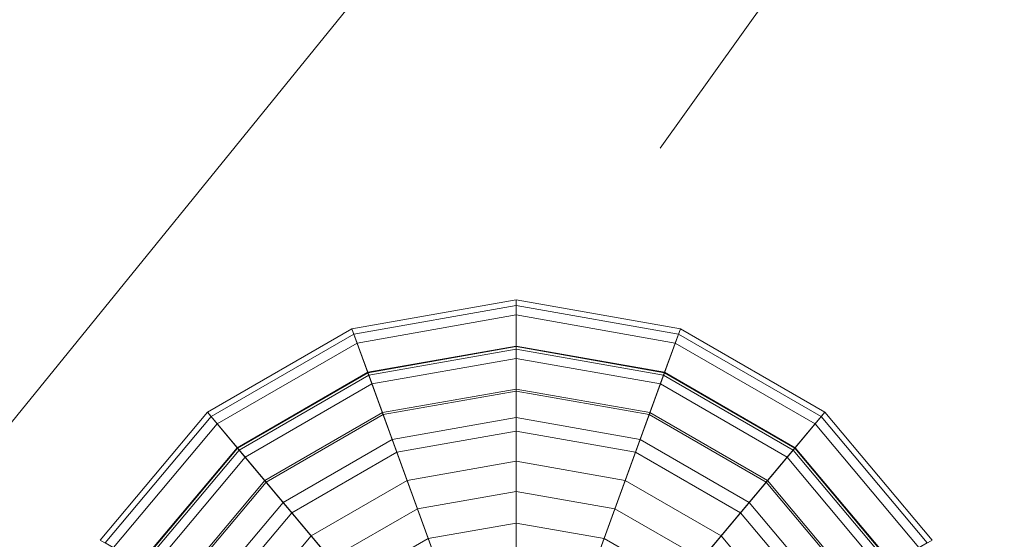
# Model space of a CAD drawing. Units: inches. Extents: x 375 to 1122, y 27 to 1069.
# Tile 15 of 155: x 728.282 to 731.058, y 269.129 to 270.593. Entities that reach past the tile are written whole.
import ezdxf

# ---------------------------------------------------------------- set-up
doc = ezdxf.new("R2010")
doc.units = ezdxf.units.IN
doc.layers.add('Furniture', color=30, linetype='Continuous', lineweight=18)

# ---------------------------------------------------------------- blocks, each defined once
blk = doc.blocks.new('A$C403C54AD')
for p, q in [((1.789224, 1.189932, 0.036628), (1.95298, 1.056939, 0.036628)), ((1.830163, 1.179702, 0.036628), (1.901807, 1.128551, 0.036628))]:
    blk.add_line(p, q)
for points in [[(1.929411, 1.147718, -0.060915), (1.946342, 1.118392, -0.057836), (1.946342, 1.118392, -0.057836), (1.920403, 1.140158, -0.060915)], [(1.931044, 1.144889, -0.057684), (1.929411, 1.147718, -0.060915), (1.920403, 1.140158, -0.060915), (1.922904, 1.138059, -0.057684)], [(1.931064, 1.144854, 0.102069), (1.929611, 1.147372, 0.088845), (1.920708, 1.139902, 0.088845), (1.922935, 1.138033, 0.102069)], [(1.929611, 1.147372, 0.088845), (1.929948, 1.146788, 0.060603), (1.921225, 1.139468, 0.060603), (1.920708, 1.139902, 0.088845)], [(1.929948, 1.146788, 0.060603), (1.932631, 1.142142, 0.042594), (1.925335, 1.13602, 0.042594), (1.921225, 1.139468, 0.060603)], [(1.939235, 1.130702, -0.054409), (1.931044, 1.144889, -0.057684), (1.922904, 1.138059, -0.057684), (1.935454, 1.127529, -0.054409)], [(1.933563, 1.140527, 0.111475), (1.931064, 1.144854, 0.102069), (1.922935, 1.138033, 0.102069), (1.926763, 1.134821, 0.111475)], [(1.931153, 1.144701, 0.088628), (1.932558, 1.142268, 0.101264), (1.925223, 1.136113, 0.101264), (1.923071, 1.137919, 0.088628)], [(1.931482, 1.144131, 0.061088), (1.931153, 1.144701, 0.088628), (1.923071, 1.137919, 0.088628), (1.923575, 1.137496, 0.061088)], [(1.934036, 1.139708, 0.043942), (1.931482, 1.144131, 0.061088), (1.923575, 1.137496, 0.061088), (1.927488, 1.134213, 0.043942)], [(1.932558, 1.142268, 0.101264), (1.935102, 1.137861, 0.111475), (1.929121, 1.132843, 0.111475), (1.925223, 1.136113, 0.101264)], [(1.932631, 1.142142, 0.042594), (1.936164, 1.136022, 0.032362), (1.930748, 1.131478, 0.032362), (1.925335, 1.13602, 0.042594)], [(1.935102, 1.137861, 0.111475), (1.933563, 1.140527, 0.111475), (1.926763, 1.134821, 0.111475), (1.929121, 1.132843, 0.111475)], [(1.920403, 1.140158, -0.060915), (1.946342, 1.118392, -0.057836), (1.946342, 1.118392, -0.057836), (1.914522, 1.129974, -0.060915)], [(1.922904, 1.138059, -0.057684), (1.920403, 1.140158, -0.060915), (1.914522, 1.129974, -0.060915), (1.917591, 1.128857, -0.057684)], [(1.922935, 1.138033, 0.102069), (1.920708, 1.139902, 0.088845), (1.914897, 1.129837, 0.088845), (1.917629, 1.128843, 0.102069)], [(1.920708, 1.139902, 0.088845), (1.921225, 1.139468, 0.060603), (1.915531, 1.129606, 0.060603), (1.914897, 1.129837, 0.088845)], [(1.921225, 1.139468, 0.060603), (1.925335, 1.13602, 0.042594), (1.920572, 1.127772, 0.042594), (1.915531, 1.129606, 0.060603)], [(1.937279, 1.134091, 0.03455), (1.934036, 1.139708, 0.043942), (1.927488, 1.134213, 0.043942), (1.932456, 1.130044, 0.03455)], [(1.935454, 1.127529, -0.054409), (1.922904, 1.138059, -0.057684), (1.917591, 1.128857, -0.057684), (1.932985, 1.123254, -0.054409)], [(1.926763, 1.134821, 0.111475), (1.922935, 1.138033, 0.102069), (1.917629, 1.128843, 0.102069), (1.922324, 1.127134, 0.111475)], [(1.923071, 1.137919, 0.088628), (1.925223, 1.136113, 0.101264), (1.920436, 1.127821, 0.101264), (1.917796, 1.128782, 0.088628)], [(1.923575, 1.137496, 0.061088), (1.923071, 1.137919, 0.088628), (1.917796, 1.128782, 0.088628), (1.918414, 1.128557, 0.061088)], [(1.927488, 1.134213, 0.043942), (1.923575, 1.137496, 0.061088), (1.918414, 1.128557, 0.061088), (1.923214, 1.12681, 0.043942)], [(1.925223, 1.136113, 0.101264), (1.929121, 1.132843, 0.111475), (1.925217, 1.126081, 0.111475), (1.920436, 1.127821, 0.101264)], [(1.925335, 1.13602, 0.042594), (1.930748, 1.131478, 0.032362), (1.927213, 1.125355, 0.032362), (1.920572, 1.127772, 0.042594)], [(1.929121, 1.132843, 0.111475), (1.926763, 1.134821, 0.111475), (1.922324, 1.127134, 0.111475), (1.925217, 1.126081, 0.111475)], [(1.932456, 1.130044, 0.03455), (1.927488, 1.134213, 0.043942), (1.923214, 1.12681, 0.043942), (1.929308, 1.124592, 0.03455)], [(1.930748, 1.131478, 0.032362), (1.938591, 1.124896, 0.024995), (1.936834, 1.121853, 0.024995), (1.927213, 1.125355, 0.032362)], [(1.939522, 1.124116, 0.027913), (1.932456, 1.130044, 0.03455), (1.929308, 1.124592, 0.03455), (1.937975, 1.121437, 0.027913)], [(1.914522, 1.129974, -0.060915), (1.946342, 1.118392, -0.057836), (1.946342, 1.118392, -0.057836), (1.91248, 1.118392, -0.060915)], [(1.917591, 1.128857, -0.057684), (1.914522, 1.129974, -0.060915), (1.91248, 1.118392, -0.060915), (1.915746, 1.118392, -0.057684)], [(1.917629, 1.128843, 0.102069), (1.914897, 1.129837, 0.088845), (1.912879, 1.118392, 0.088845), (1.915786, 1.118392, 0.102069)], [(1.914897, 1.129837, 0.088845), (1.915531, 1.129606, 0.060603), (1.913554, 1.118392, 0.060603), (1.912879, 1.118392, 0.088845)], [(1.915531, 1.129606, 0.060603), (1.920572, 1.127772, 0.042594), (1.918919, 1.118392, 0.042594), (1.913554, 1.118392, 0.060603)], [(1.932985, 1.123254, -0.054409), (1.917591, 1.128857, -0.057684), (1.915746, 1.118392, -0.057684), (1.932128, 1.118392, -0.054409)], [(1.922324, 1.127134, 0.111475), (1.917629, 1.128843, 0.102069), (1.915786, 1.118392, 0.102069), (1.920783, 1.118392, 0.111475)], [(1.917796, 1.128782, 0.088628), (1.920436, 1.127821, 0.101264), (1.918773, 1.118392, 0.101264), (1.915964, 1.118392, 0.088628)], [(1.918414, 1.128557, 0.061088), (1.917796, 1.128782, 0.088628), (1.915964, 1.118392, 0.088628), (1.916622, 1.118392, 0.061088)], [(1.923214, 1.12681, 0.043942), (1.918414, 1.128557, 0.061088), (1.916622, 1.118392, 0.061088), (1.921729, 1.118392, 0.043942)], [(1.920436, 1.127821, 0.101264), (1.925217, 1.126081, 0.111475), (1.923861, 1.118392, 0.111475), (1.918773, 1.118392, 0.101264)], [(1.920572, 1.127772, 0.042594), (1.927213, 1.125355, 0.032362), (1.925985, 1.118392, 0.032362), (1.918919, 1.118392, 0.042594)], [(1.925217, 1.126081, 0.111475), (1.922324, 1.127134, 0.111475), (1.920783, 1.118392, 0.111475), (1.923861, 1.118392, 0.111475)], [(1.929308, 1.124592, 0.03455), (1.923214, 1.12681, 0.043942), (1.921729, 1.118392, 0.043942), (1.928215, 1.118392, 0.03455)], [(1.927213, 1.125355, 0.032362), (1.936834, 1.121853, 0.024995), (1.936224, 1.118392, 0.024995), (1.925985, 1.118392, 0.032362)], [(1.937975, 1.121437, 0.027913), (1.929308, 1.124592, 0.03455), (1.928215, 1.118392, 0.03455), (1.937438, 1.118392, 0.027913)], [(1.91248, 1.118392, -0.060915), (1.946342, 1.118392, -0.057836), (1.946342, 1.118392, -0.057836), (1.914522, 1.106811, -0.060915)], [(1.915746, 1.118392, -0.057684), (1.91248, 1.118392, -0.060915), (1.914522, 1.106811, -0.060915), (1.917591, 1.107928, -0.057684)], [(1.915786, 1.118392, 0.102069), (1.912879, 1.118392, 0.088845), (1.914897, 1.106947, 0.088845), (1.917629, 1.107941, 0.102069)], [(1.912879, 1.118392, 0.088845), (1.913554, 1.118392, 0.060603), (1.915531, 1.107178, 0.060603), (1.914897, 1.106947, 0.088845)], [(1.913554, 1.118392, 0.060603), (1.918919, 1.118392, 0.042594), (1.920572, 1.109013, 0.042594), (1.915531, 1.107178, 0.060603)], [(1.914522, 1.106811, -0.060915), (1.946342, 1.118392, -0.057836), (1.946342, 1.118392, -0.057836), (1.920403, 1.096626, -0.060915)], [(1.932128, 1.118392, -0.054409), (1.915746, 1.118392, -0.057684), (1.917591, 1.107928, -0.057684), (1.932985, 1.113531, -0.054409)], [(1.920783, 1.118392, 0.111475), (1.915786, 1.118392, 0.102069), (1.917629, 1.107941, 0.102069), (1.922324, 1.10965, 0.111475)], [(1.915964, 1.118392, 0.088628), (1.918773, 1.118392, 0.101264), (1.920436, 1.108963, 0.101264), (1.917796, 1.108002, 0.088628)], [(1.916622, 1.118392, 0.061088), (1.915964, 1.118392, 0.088628), (1.917796, 1.108002, 0.088628), (1.918414, 1.108227, 0.061088)], [(1.921729, 1.118392, 0.043942), (1.916622, 1.118392, 0.061088), (1.918414, 1.108227, 0.061088), (1.923214, 1.109974, 0.043942)], [(1.918773, 1.118392, 0.101264), (1.923861, 1.118392, 0.111475), (1.925217, 1.110703, 0.111475), (1.920436, 1.108963, 0.101264)], [(1.918919, 1.118392, 0.042594), (1.925985, 1.118392, 0.032362), (1.927213, 1.111429, 0.032362), (1.920572, 1.109013, 0.042594)], [(1.920403, 1.096626, -0.060915), (1.946342, 1.118392, -0.057836), (1.946342, 1.118392, -0.057836), (1.929411, 1.089067, -0.060915)], [(1.923861, 1.118392, 0.111475), (1.920783, 1.118392, 0.111475), (1.922324, 1.10965, 0.111475), (1.925217, 1.110703, 0.111475)], [(1.928215, 1.118392, 0.03455), (1.921729, 1.118392, 0.043942), (1.923214, 1.109974, 0.043942), (1.929308, 1.112192, 0.03455)], [(1.925985, 1.118392, 0.032362), (1.936224, 1.118392, 0.024995), (1.936834, 1.114931, 0.024995), (1.927213, 1.111429, 0.032362)], [(1.937438, 1.118392, 0.027913), (1.928215, 1.118392, 0.03455), (1.929308, 1.112192, 0.03455), (1.937975, 1.115347, 0.027913)], [(1.927213, 1.111429, 0.032362), (1.936834, 1.114931, 0.024995), (1.938591, 1.111888, 0.024995), (1.930748, 1.105307, 0.032362)], [(1.937975, 1.115347, 0.027913), (1.929308, 1.112192, 0.03455), (1.932456, 1.10674, 0.03455), (1.939522, 1.112669, 0.027913)], [(1.932985, 1.113531, -0.054409), (1.917591, 1.107928, -0.057684), (1.922904, 1.098725, -0.057684), (1.935454, 1.109255, -0.054409)], [(1.929308, 1.112192, 0.03455), (1.923214, 1.109974, 0.043942), (1.927488, 1.102571, 0.043942), (1.932456, 1.10674, 0.03455)], [(1.920572, 1.109013, 0.042594), (1.927213, 1.111429, 0.032362), (1.930748, 1.105307, 0.032362), (1.925335, 1.100764, 0.042594)], [(1.920436, 1.108963, 0.101264), (1.925217, 1.110703, 0.111475), (1.929121, 1.103941, 0.111475), (1.925223, 1.100671, 0.101264)], [(1.925217, 1.110703, 0.111475), (1.922324, 1.10965, 0.111475), (1.926763, 1.101963, 0.111475), (1.929121, 1.103941, 0.111475)], [(1.923214, 1.109974, 0.043942), (1.918414, 1.108227, 0.061088), (1.923575, 1.099288, 0.061088), (1.927488, 1.102571, 0.043942)], [(1.922324, 1.10965, 0.111475), (1.917629, 1.107941, 0.102069), (1.922935, 1.098751, 0.102069), (1.926763, 1.101963, 0.111475)], [(1.935454, 1.109255, -0.054409), (1.922904, 1.098725, -0.057684), (1.931044, 1.091895, -0.057684), (1.939235, 1.106082, -0.054409)], [(1.915531, 1.107178, 0.060603), (1.920572, 1.109013, 0.042594), (1.925335, 1.100764, 0.042594), (1.921225, 1.097316, 0.060603)], [(1.917796, 1.108002, 0.088628), (1.920436, 1.108963, 0.101264), (1.925223, 1.100671, 0.101264), (1.923071, 1.098865, 0.088628)], [(1.917591, 1.107928, -0.057684), (1.914522, 1.106811, -0.060915), (1.920403, 1.096626, -0.060915), (1.922904, 1.098725, -0.057684)], [(1.917629, 1.107941, 0.102069), (1.914897, 1.106947, 0.088845), (1.920708, 1.096882, 0.088845), (1.922935, 1.098751, 0.102069)], [(1.918414, 1.108227, 0.061088), (1.917796, 1.108002, 0.088628), (1.923071, 1.098865, 0.088628), (1.923575, 1.099288, 0.061088)], [(1.914897, 1.106947, 0.088845), (1.915531, 1.107178, 0.060603), (1.921225, 1.097316, 0.060603), (1.920708, 1.096882, 0.088845)], [(1.932456, 1.10674, 0.03455), (1.927488, 1.102571, 0.043942), (1.934036, 1.097077, 0.043942), (1.937279, 1.102693, 0.03455)], [(1.925335, 1.100764, 0.042594), (1.930748, 1.105307, 0.032362), (1.936164, 1.100762, 0.032362), (1.932631, 1.094642, 0.042594)], [(1.925223, 1.100671, 0.101264), (1.929121, 1.103941, 0.111475), (1.935102, 1.098923, 0.111475), (1.932558, 1.094517, 0.101264)], [(1.929121, 1.103941, 0.111475), (1.926763, 1.101963, 0.111475), (1.933563, 1.096257, 0.111475), (1.935102, 1.098923, 0.111475)], [(1.927488, 1.102571, 0.043942), (1.923575, 1.099288, 0.061088), (1.931482, 1.092653, 0.061088), (1.934036, 1.097077, 0.043942)], [(1.926763, 1.101963, 0.111475), (1.922935, 1.098751, 0.102069), (1.931064, 1.09193, 0.102069), (1.933563, 1.096257, 0.111475)], [(1.921225, 1.097316, 0.060603), (1.925335, 1.100764, 0.042594), (1.932631, 1.094642, 0.042594), (1.929948, 1.089997, 0.060603)], [(1.923071, 1.098865, 0.088628), (1.925223, 1.100671, 0.101264), (1.932558, 1.094517, 0.101264), (1.931153, 1.092083, 0.088628)], [(1.923575, 1.099288, 0.061088), (1.923071, 1.098865, 0.088628), (1.931153, 1.092083, 0.088628), (1.931482, 1.092653, 0.061088)], [(1.922904, 1.098725, -0.057684), (1.920403, 1.096626, -0.060915), (1.929411, 1.089067, -0.060915), (1.931044, 1.091895, -0.057684)], [(1.922935, 1.098751, 0.102069), (1.920708, 1.096882, 0.088845), (1.929611, 1.089412, 0.088845), (1.931064, 1.09193, 0.102069)], [(1.920708, 1.096882, 0.088845), (1.921225, 1.097316, 0.060603), (1.929948, 1.089997, 0.060603), (1.929611, 1.089412, 0.088845)]]:
    blk.add_3dface(points)

msp = doc.modelspace()

# ---------------------------------------------------------------- block references
at = {"layer": 'Furniture', "xscale": 39.9918517141215, "yscale": 39.9918517141215, "zscale": 39.9918517141215, "rotation": 270}
msp.add_blockref('A$C403C54AD', (684.9549, 346.2875, 0.024), dxfattribs=at)

doc.saveas('drawing.dxf')
